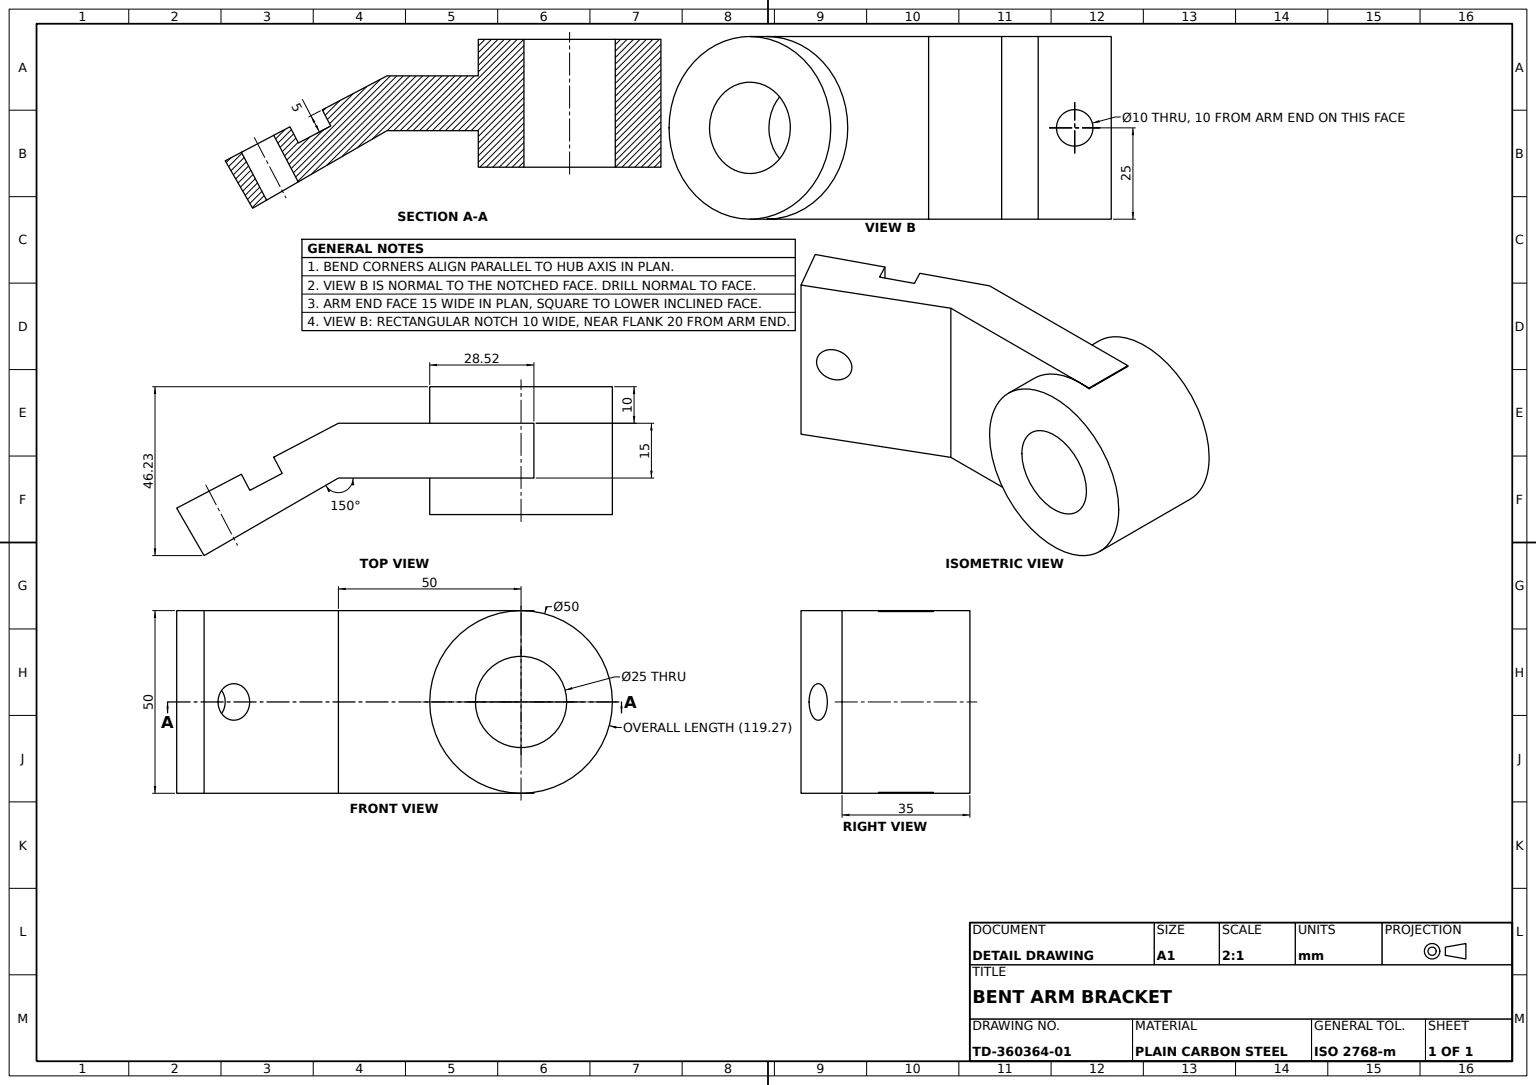
SolidWorks part; units mm, degrees
material "Plain Carbon Steel"
ref_plane "Front Plane" through (0, 0, 0) normal (0, 0, 1) x (1, 0, 0)
ref_plane "Top Plane" through (0, 0, 0) normal (0, 1, 0) x (1, 0, 0)
ref_plane "Right Plane" through (0, 0, 0) normal (1, 0, 0) x (0, 0, -1)
sketch "Hub Tube Sketch Ø50-Ø25" plane through (0, 0, 0) normal (0, 0, 1) x (1, 0, 0)
  circle A0 centre (0, 0) radius 12.5
  circle A1 centre (0, 0) radius 25
  dimension "D1" = 25
  dimension "D2" = 50
extrude "Hub Tube Ø50-Ø25 x35" add sketch "Hub Tube Sketch Ø50-Ø25" along normal mid plane 35
sketch "Arm Profile Sketch" plane through (0, 0, 0) normal (0, 1, 0) x (1, 0, 0)
  line L0 (0, 0) -> (-63.0652, 0) construction
  line L1 (-25, 0) -> (-50, 0)
  line L2 (-25, 17.5) -> (-25, -17.5) construction
  line L3 (-25, 7.5) -> (-50, 7.5)
  line L4 (-25, -7.5) -> (-50, -7.5)
  line L5 (-50, -7.5) -> (-86.7711, -28.7298)
  line L6 (-86.7711, -28.7298) -> (-94.2711, -15.7394)
  line L7 (-94.2711, -15.7394) -> (-50, 7.5)
  line L8 (-25, 7.5) -> (3.5206, 7.5)
  line L9 (3.5206, 7.5) -> (3.5206, -7.5)
  line L10 (3.5206, -7.5) -> (-25, -7.5)
  dimension "D1" = 25
  dimension "D4" = 15
  dimension "D5" = 50
  dimension "D6" = 150
  dimension "D7" = 28.5206
  dimension "D2" = 7.5
  dimension "D3" = 7.5
extrude "Arm 50" add sketch "Arm Profile Sketch" along normal mid plane 50
sketch "Top Notch Sketch" plane through (0, 25, 0) normal (0, 1, 0) x (1, 0, 0)
  line L0 (-76.5627, -6.4437) -> (-74.2387, -10.8708)
  line L1 (-94.2711, -15.7394) -> (-50, 7.5) construction
  line L2 (-74.2387, -10.8708) -> (-65.3845, -6.2229)
  line L3 (-65.3845, -6.2229) -> (-67.7084, -1.7958)
  line L4 (-76.5627, -6.4437) -> (-67.7084, -1.7958)
  dimension "D1" = 20
  dimension "D2" = 10
  dimension "D3" = 5
extrude "Top Notch Cut" cut sketch "Top Notch Sketch" against normal through all
sketch "Cross Hole Sketch Ø10" plane through (-13.8879, 0, -26.4565) normal (-0.4648, 0, -0.8854) x (-0.8854, 0, 0.4648)
  line L0 (90.7852, 0) -> (80.7852, 0) construction
  line L1 (90.7852, 25) -> (90.7852, -25) construction
  circle A0 centre (80.7852, 0) radius 5
  dimension "D2" = 10
  dimension "D1" = 10
extrude "Cross Hole Ø10" cut sketch "Cross Hole Sketch Ø10" against normal through all
sketch "Bore Clearance Sketch" plane through (0, 0, -17.5) normal (0, 0, -1) x (-1, 0, 0)
  line L0 (-3.5206, 11.994) -> (-3.5206, -11.994) construction
  line L1 (-3.5206, 11.994) -> (-3.5206, -11.994)
  arc A0 (-3.5206, -11.994) -> (-3.5206, 11.994) centre (0, 0) ccw construction
  arc A1 (-3.5206, -11.994) -> (-3.5206, 11.994) centre (0, 0) ccw
extrude "Bore Clearance Cut" cut sketch "Bore Clearance Sketch" against normal through all
